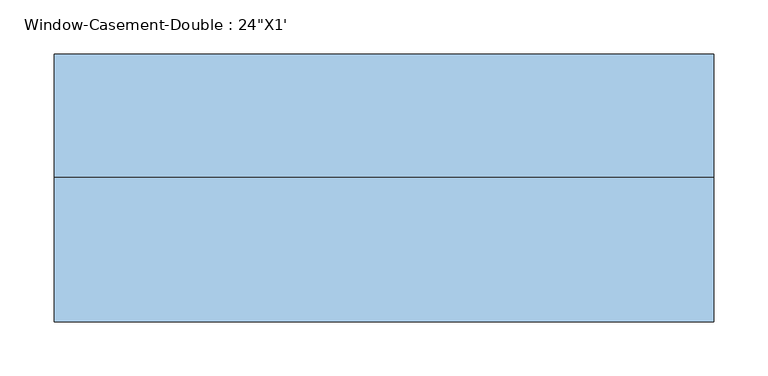
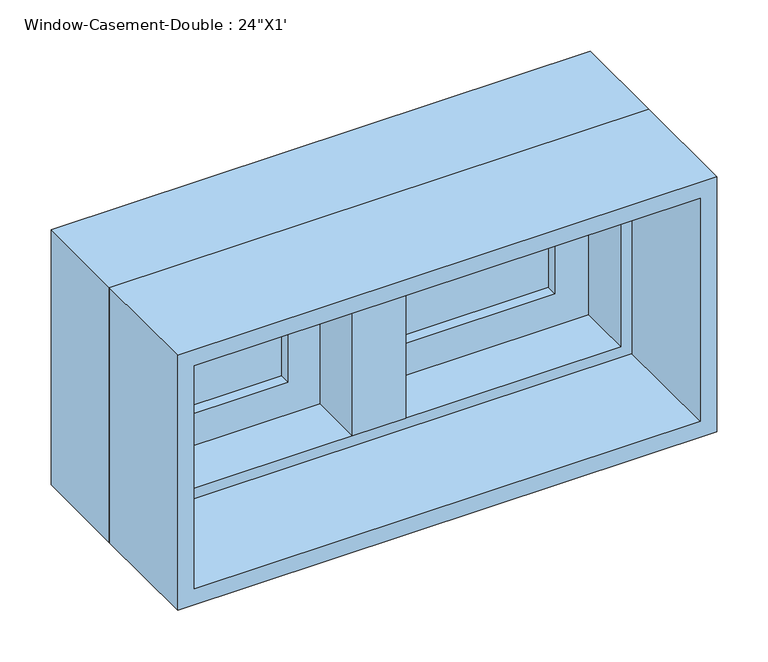
"""IFC4 building model written with IfcOpenShell, lengths in millimetres: window geometry."""

from ifc_helpers import new_model, si_unit, frame, origin, place, context, project, spatial, polyline, outline, extrude, faceted_brep, source, transform, mapped, element, save


def window_375d1de9(model_context):
    return source(origin(), model_context, "Body", "SolidModel", [
        faceted_brep([(9.525, 133.35, 1206.5), (-9.525, 133.35, 1206.5), (-9.525, 82.55, 1206.5), (9.525, 82.55, 1206.5), (9.525, 133.35, 927.1), (9.525, 82.55, 927.1), (-9.525, 82.55, 927.1), (-9.525, 133.35, 927.1), (-9.525, 82.55, 946.15), (-9.525, 82.55, 1187.45), (-30.1625, 82.55, 946.15), (-30.1625, 82.55, 1187.45), (-30.1625, 19.05, 946.15), (-30.1625, 19.05, 1187.45), (30.1625, 19.05, 946.15), (30.1625, 19.05, 1187.45), (30.1625, 82.55, 946.15), (30.1625, 82.55, 1187.45), (9.525, 82.55, 946.15), (9.525, 82.55, 1187.45)], [[[0, 1, 2, 3]], [[4, 5, 6, 7]], [[1, 0, 4, 7]], [[2, 1, 7, 6, 8, 9]], [[9, 8, 10, 11]], [[11, 10, 12, 13]], [[13, 12, 14, 15]], [[15, 14, 16, 17]], [[17, 16, 18, 19]], [[0, 3, 19, 18, 5, 4]], [[18, 8, 6, 5]], [[9, 19, 3, 2]], [[8, 18, 16, 14, 12, 10]], [[19, 9, 11, 13, 15, 17]]]),
        extrude(outline(polyline([(-66.675, 114.3), (-66.675, 107.95), (-234.95, 107.95), (-234.95, 114.3), (-66.675, 114.3)])), frame((0.0, 0.0, 984.25), z_axis=(0.0, 0.0, 1.0), x_axis=(1.0, 0.0, 0.0)), (0.0, 0.0, 1.0), 165.1),
        extrude(outline(polyline([(-234.95, 95.25), (-234.95, 101.6), (-66.675, 101.6), (-66.675, 95.25), (-234.95, 95.25)])), frame((0.0, 0.0, 984.25), z_axis=(0.0, 0.0, 1.0), x_axis=(1.0, 0.0, 0.0)), (0.0, 0.0, 1.0), 165.1),
        extrude(outline(polyline([(234.95, 114.3), (234.95, 107.95), (66.675, 107.95), (66.675, 114.3), (234.95, 114.3)])), frame((0.0, 0.0, 984.25), z_axis=(0.0, 0.0, 1.0), x_axis=(1.0, 0.0, 0.0)), (0.0, 0.0, 1.0), 165.1),
        extrude(outline(polyline([(66.675, 95.25), (66.675, 101.6), (234.95, 101.6), (234.95, 95.25), (66.675, 95.25)])), frame((0.0, 0.0, 984.25), z_axis=(0.0, 0.0, 1.0), x_axis=(1.0, 0.0, 0.0)), (0.0, 0.0, 1.0), 165.1),
        extrude(outline(polyline([(1206.5, -292.1), (927.1, -292.1), (927.1, -9.525), (1206.5, -9.525), (1206.5, -292.1)]), holes=[polyline([(1149.35, -66.675), (984.25, -66.675), (984.25, -234.95), (1149.35, -234.95), (1149.35, -66.675)])]), frame((0.0, 82.55, 0.0), z_axis=(0.0, 1.0, 0.0), x_axis=(0.0, 0.0, 1.0)), (0.0, 0.0, 1.0), 44.45),
        extrude(outline(polyline([(927.1, 292.1), (1206.5, 292.1), (1206.5, 9.525), (927.1, 9.525), (927.1, 292.1)]), holes=[polyline([(984.25, 66.675), (1149.35, 66.675), (1149.35, 234.95), (984.25, 234.95), (984.25, 66.675)])]), frame((0.0, 82.55, 0.0), z_axis=(0.0, 1.0, 0.0), x_axis=(0.0, 0.0, 1.0)), (0.0, 0.0, 1.0), 44.45),
        extrude(outline(polyline([(1219.2, -304.8), (914.4, -304.8), (914.4, 304.8), (1219.2, 304.8), (1219.2, -304.8)]), holes=[polyline([(1200.15, 285.75), (933.45, 285.75), (933.45, -285.75), (1200.15, -285.75), (1200.15, 285.75)])]), frame((0.0, -114.3, 0.0), z_axis=(0.0, 1.0, 0.0), x_axis=(0.0, 0.0, 1.0)), (0.0, 0.0, 1.0), 133.35),
        faceted_brep([(273.05, 82.55, 1187.45), (273.05, 19.05, 1187.45), (-273.05, 19.05, 1187.45), (-273.05, 82.55, 1187.45), (292.1, 133.35, 1206.5), (292.1, 82.55, 1206.5), (-292.1, 82.55, 1206.5), (-292.1, 133.35, 1206.5), (304.8, 19.05, 1219.2), (304.8, 133.35, 1219.2), (-304.8, 133.35, 1219.2), (-304.8, 19.05, 1219.2), (-273.05, 19.05, 946.15), (-273.05, 82.55, 946.15), (-292.1, 82.55, 927.1), (-292.1, 133.35, 927.1), (-304.8, 133.35, 914.4), (-304.8, 19.05, 914.4), (273.05, 19.05, 946.15), (273.05, 82.55, 946.15), (292.1, 82.55, 927.1), (292.1, 133.35, 927.1), (304.8, 133.35, 914.4), (304.8, 19.05, 914.4)], [[[0, 1, 2, 3]], [[4, 5, 6, 7]], [[8, 9, 10, 11]], [[3, 2, 12, 13]], [[7, 6, 14, 15]], [[11, 10, 16, 17]], [[13, 12, 18, 19]], [[15, 14, 20, 21]], [[17, 16, 22, 23]], [[11, 17, 23, 8], [1, 18, 12, 2]], [[19, 18, 1, 0]], [[5, 20, 14, 6], [3, 13, 19, 0]], [[21, 20, 5, 4]], [[23, 22, 9, 8]], [[9, 22, 16, 10], [7, 15, 21, 4]]]),
    ])


if __name__ == "__main__":
    model = new_model("IFC4")
    model_context = context("Model", 3, world=origin())
    ifc_project = project(units=[si_unit("LENGTHUNIT", "METRE", prefix="MILLI")], contexts=[model_context])
    site = spatial("IfcSite", under=ifc_project)
    building = spatial("IfcBuilding", under=site)
    placement = place(None, origin())
    window_shape = window_375d1de9(model_context)
    element("IfcWindow", 1, ObjectType="Window-Casement-Double : 24\"X1'", at=placement, inside=building, context=model_context, shape_type="MappedRepresentation", body=[
        mapped(window_shape, transform((0.0, 0.0, 0.0), x_axis=(1.0, 0.0, 0.0), y_axis=(0.0, 1.0, 0.0), z_axis=(0.0, 0.0, 1.0))),
    ])
    save(model, "model.ifc")

# Revit data of these elements
# Type "Window-Casement-Double : 24\"X1'"
#   Type Mark = "V"
#   Fire Rating = "0.5h"
#   Assembly Code = "B2020100"
#   Analytic Construction = "Double glazing - domestic"
#   Frame Extension [instance default] = 0' - 0 1/4"
#   Window Inset [instance default] = 0' - 0"
#   Wall Thickness [instance default] = 0' - 6"
#   Interior Wall Closure [instance default] = 0' - 2 1/4"
#   Half Width = 1' - 0"
#   Visual Light Transmittance = 0.81
#   Thermal Resistance (R) = 1.8146 (h·ft²·°F)/BTU
#   Solar Heat Gain Coefficient = 0.76
#   Rough Width = 2' - 0 1/2"
#   Rough Height = 1' - 0 1/2"
#   Height = 1' - 0"
#   Heat Transfer Coefficient (U) = 0.5511 BTU/(h·ft²·°F)
#   Exterior Wall Closure [instance default] = 0' - 1 1/4"
#   Extension Jamb [instance default] = 0' - 2 1/4"
#   Default Sill Height = 3' - 0"
#   Width = 2' - 0"
#   Muntin Visibility = yes
#   Interior Trim Visibility [instance default] = yes
#   Exterior Trim Visibility [instance default] = yes
#   Extension Jamb Visibility [instance default] = yes
#   Interior Trim Material = Wood - Stained
#   Muntin Pattern = Muntin Pattern_2x2 : Muntin Pattern_2x2
#   Interior Trim = Trim-Window-Interior-Flat : Picture Frame
#   Interior Frame Material = Wood - Stained
#   Glass Panel Material = Glass
#   Exterior Trim Material = Clad - White
#   Exterior Trim = Trim-Window-Exterior-Flat : with Sill
#   Exterior Frame Material = Clad - White
#   Wall Closure = (empty or 0)
# Element 1 (IfcWindow, "Window-Casement-Double : 24\"X1'")
#   Wall Thickness = 0' - 9"
#   Extension Jamb = 0' - 5 1/4"
#   Materials on its faces: "Wood - Stained", "Glass", "Clad - White"
# Materials
#   "Wood - Stained": class "Wood", colour RGB 224 178 126, transparency 0, Cost = 0
#   "Glass": class "Glass", colour RGB 0 128 192, transparency 0.75, Description = "Soda Lime Glass", Cost = 0
#   "Clad - White": class "Wood", colour RGB 242 242 238, transparency 0, Cost = 0
